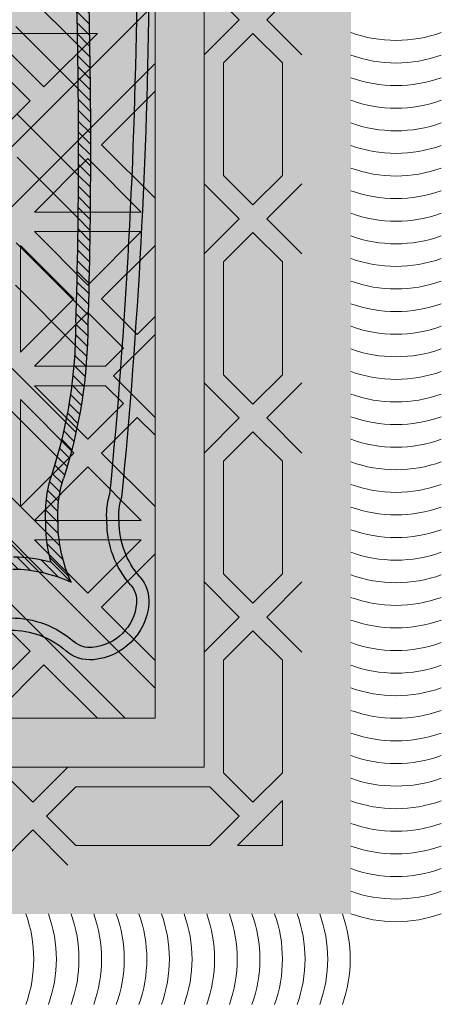
# Model space of a CAD drawing. Units: inches. Extents: x 844 to 2234, y 346 to 1084.
# Tile 29 of 93: x 1260.07 to 1265.57, y 682.93 to 695.76. Entities that reach past the tile are written whole.
import ezdxf

# ---------------------------------------------------------------- set-up
doc = ezdxf.new("R2010")
doc.units = ezdxf.units.IN
doc.header["$MEASUREMENT"] = 0
doc.layers.add('furniture', color=8, linetype='Continuous', lineweight=18)
doc.layers.add('RA-AP-01$0$INT', color=35, linetype='Continuous', lineweight=5)
doc.layers.add('RA-AP-01$0$FURN', color=3, linetype='Continuous')
doc.layers.add('RA-AP-01$0$WOOD', color=64, linetype='Continuous')

# ---------------------------------------------------------------- blocks, each defined once
blk = doc.blocks.new('A$C18D01794')
at = {"layer": 'RA-AP-01$0$INT'}
h = blk.add_hatch(color=256, dxfattribs=at)
h.paths.add_polyline_path([(4.3552, -6.1567), (4.3552, -8.0567), (5.4552, -8.0567), (5.4552, -6.1567)])
h.paths.add_polyline_path([(4.4052, -8.0067), (4.4052, -6.2067), (5.4052, -6.2067), (5.4052, -8.0067)], flags=16)
h = blk.add_hatch(color=256, dxfattribs=at)
h.paths.add_polyline_path([(4.4693, -7.0709), (4.5052, -7.035), (4.5052, -7.1067)])
h.paths.add_polyline_path([(4.4552, -7.085), (4.4769, -7.1067), (4.4335, -7.1067)])
h.paths.add_polyline_path([(4.4052, -7.035), (4.4411, -7.0709), (4.4052, -7.1067)])
h.paths.add_polyline_path([(4.4252, -6.9115), (4.4552, -6.8815), (4.4852, -6.9115), (4.4852, -7.0267), (4.4552, -7.0567), (4.4252, -7.0267)])
h.paths.add_polyline_path([(4.5052, -6.8315), (4.5052, -6.9032), (4.4693, -6.8673)])
h.paths.add_polyline_path([(4.4252, -6.7079), (4.4552, -6.6779), (4.4852, -6.7079), (4.4852, -6.8232), (4.4552, -6.8532), (4.4252, -6.8232)])
h.paths.add_polyline_path([(4.4252, -6.5044), (4.4552, -6.4744), (4.4852, -6.5044), (4.4852, -6.6196), (4.4552, -6.6496), (4.4252, -6.6196)])
h.paths.add_polyline_path([(4.4693, -6.6638), (4.5052, -6.6279), (4.5052, -6.6996)])
h.paths.add_polyline_path([(4.4052, -6.6279), (4.4411, -6.6638), (4.4052, -6.6996)])
h.paths.add_polyline_path([(4.4052, -6.4244), (4.4411, -6.4602), (4.4052, -6.4961)])
h.paths.add_polyline_path([(4.4693, -6.4602), (4.5052, -6.4244), (4.5052, -6.4961)])
h.paths.add_polyline_path([(4.4252, -6.3009), (4.4552, -6.2709), (4.4852, -6.3009), (4.4852, -6.4161), (4.4552, -6.4461), (4.4252, -6.4161)])
h.paths.add_polyline_path([(4.4252, -6.2267), (4.4711, -6.2267), (4.4252, -6.2726)])
h.paths.add_polyline_path([(4.4993, -6.2267), (4.6361, -6.2267), (4.6661, -6.2567), (4.6361, -6.2867), (4.4993, -6.2867), (4.4693, -6.2567)])
h.paths.add_polyline_path([(4.6802, -6.2709), (4.7161, -6.3067), (4.6443, -6.3067)])
h.paths.add_polyline_path([(4.6443, -6.2067), (4.7161, -6.2067), (4.6802, -6.2426)])
h.paths.add_polyline_path([(4.7243, -6.2267), (4.8611, -6.2267), (4.8911, -6.2567), (4.8611, -6.2867), (4.7243, -6.2867), (4.6943, -6.2567)])
h.paths.add_polyline_path([(4.9052, -6.2709), (4.9411, -6.3067), (4.8693, -6.3067)])
h.paths.add_polyline_path([(4.8693, -6.2067), (4.9411, -6.2067), (4.9052, -6.2426)])
h.paths.add_polyline_path([(4.9493, -6.2267), (5.0861, -6.2267), (5.1161, -6.2567), (5.0861, -6.2867), (4.9493, -6.2867), (4.9193, -6.2567)])
h.paths.add_polyline_path([(5.1302, -6.2709), (5.1661, -6.3067), (5.0943, -6.3067)])
h.paths.add_polyline_path([(5.0943, -6.2067), (5.1661, -6.2067), (5.1302, -6.2426)])
h.paths.add_polyline_path([(5.1743, -6.2267), (5.3111, -6.2267), (5.3411, -6.2567), (5.3111, -6.2867), (5.1743, -6.2867), (5.1443, -6.2567)])
h.paths.add_polyline_path([(5.3252, -6.3009), (5.3552, -6.2709), (5.3852, -6.3009), (5.3852, -6.4161), (5.3552, -6.4461), (5.3252, -6.4161)])
h.paths.add_polyline_path([(5.3393, -6.2267), (5.3852, -6.2267), (5.3852, -6.2726)])
h.paths.add_polyline_path([(5.3252, -6.5044), (5.3552, -6.4744), (5.3852, -6.5044), (5.3852, -6.6196), (5.3552, -6.6496), (5.3252, -6.6196)])
h.paths.add_polyline_path([(5.3052, -6.4244), (5.3411, -6.4602), (5.3052, -6.4961)])
h.paths.add_polyline_path([(5.3693, -6.4602), (5.4052, -6.4244), (5.4052, -6.4961)])
h.paths.add_polyline_path([(5.4052, -6.6279), (5.4052, -6.6996), (5.3693, -6.6638)])
h.paths.add_polyline_path([(5.3052, -6.6279), (5.3411, -6.6638), (5.3052, -6.6996)])
h.paths.add_polyline_path([(5.3252, -6.7079), (5.3552, -6.6779), (5.3852, -6.7079), (5.3852, -6.8232), (5.3552, -6.8532), (5.3252, -6.8232)])
h.paths.add_polyline_path([(5.3052, -6.8315), (5.3411, -6.8673), (5.3052, -6.9032)])
h.paths.add_polyline_path([(5.3252, -6.9115), (5.3552, -6.8815), (5.3852, -6.9115), (5.3852, -7.0267), (5.3552, -7.0567), (5.3252, -7.0267)])
h.paths.add_polyline_path([(5.4046, -6.8321, 0.001218), (5.4052, -6.8323), (5.4052, -6.9032), (5.3693, -6.8673)])
h.paths.add_polyline_path([(5.3693, -7.0709), (5.4052, -7.035), (5.4052, -7.1067)])
h.paths.add_polyline_path([(5.3552, -7.085), (5.3769, -7.1067), (5.3335, -7.1067)])
h.paths.add_polyline_path([(5.3052, -7.035), (5.3411, -7.0709), (5.3052, -7.1067)])
h = blk.add_hatch(color=256, dxfattribs=at)
h.paths.add_polyline_path([(4.5052, -6.6279), (4.4693, -6.6638), (4.5052, -6.6996), (4.5052, -6.8315), (4.4693, -6.8673), (4.5052, -6.9032), (4.5052, -7.035), (4.4693, -7.0709), (4.5052, -7.1067), (4.4769, -7.1067), (4.4552, -7.085), (4.4335, -7.1067), (4.4052, -7.1067), (4.4411, -7.0709), (4.4052, -7.035), (4.4052, -6.9032), (4.4411, -6.8673), (4.4052, -6.8315), (4.4052, -6.6996), (4.4411, -6.6638), (4.4052, -6.6279), (4.4052, -6.4961), (4.4411, -6.4602), (4.4052, -6.4244), (4.4052, -6.2067), (4.6443, -6.2067), (4.6802, -6.2426), (4.7161, -6.2067), (4.8693, -6.2067), (4.9052, -6.2426), (4.9411, -6.2067), (5.0943, -6.2067), (5.1302, -6.2426), (5.1661, -6.2067), (5.4052, -6.2067), (5.4052, -6.4244), (5.3693, -6.4602), (5.4052, -6.4961), (5.4052, -6.6279), (5.3693, -6.6638), (5.4052, -6.6996), (5.4052, -6.8315), (5.3693, -6.8673), (5.4052, -6.9032), (5.4052, -7.035), (5.3693, -7.0709), (5.4052, -7.1067), (5.3769, -7.1067), (5.3552, -7.085), (5.3335, -7.1067), (5.3052, -7.1067), (5.3411, -7.0709), (5.3052, -7.035), (5.3052, -6.9032), (5.3411, -6.8673), (5.3052, -6.8315), (5.3052, -6.6996), (5.3411, -6.6638), (5.3052, -6.6279), (5.3052, -6.4961), (5.3411, -6.4602), (5.3052, -6.4244), (5.3052, -6.3067), (5.1661, -6.3067), (5.1302, -6.2709), (5.0943, -6.3067), (4.9411, -6.3067), (4.9052, -6.2709), (4.8693, -6.3067), (4.7161, -6.3067), (4.6802, -6.2709), (4.6443, -6.3067), (4.5052, -6.3067), (4.5052, -6.4244), (4.4693, -6.4602), (4.5052, -6.4961)])
h.paths.add_polyline_path([(4.4852, -6.5044), (4.4552, -6.4744), (4.4252, -6.5044), (4.4252, -6.6196), (4.4552, -6.6496), (4.4852, -6.6196)], flags=16)
h.paths.add_polyline_path([(4.4552, -6.4461), (4.4852, -6.4161), (4.4852, -6.3009), (4.4552, -6.2709), (4.4252, -6.3009), (4.4252, -6.4161)], flags=16)
h.paths.add_polyline_path([(4.4552, -6.6779), (4.4252, -6.7079), (4.4252, -6.8232), (4.4552, -6.8532), (4.4852, -6.8232), (4.4852, -6.7079)], flags=16)
h.paths.add_polyline_path([(4.4993, -6.2867), (4.6361, -6.2867), (4.6661, -6.2567), (4.6361, -6.2267), (4.4993, -6.2267), (4.4693, -6.2567)], flags=16)
h.paths.add_polyline_path([(4.4252, -6.2726), (4.4711, -6.2267), (4.4252, -6.2267)], flags=16)
h.paths.add_polyline_path([(4.4552, -6.8815), (4.4252, -6.9115), (4.4252, -7.0267), (4.4552, -7.0567), (4.4852, -7.0267), (4.4852, -6.9115)], flags=16)
h.paths.add_polyline_path([(4.7243, -6.2867), (4.8611, -6.2867), (4.8911, -6.2567), (4.8611, -6.2267), (4.7243, -6.2267), (4.6943, -6.2567)], flags=16)
h.paths.add_polyline_path([(4.9193, -6.2567), (4.9493, -6.2867), (5.0861, -6.2867), (5.1161, -6.2567), (5.0861, -6.2267), (4.9493, -6.2267)], flags=16)
h.paths.add_polyline_path([(5.1443, -6.2567), (5.1743, -6.2867), (5.3111, -6.2867), (5.3411, -6.2567), (5.3111, -6.2267), (5.1743, -6.2267)], flags=16)
h.paths.add_polyline_path([(5.3252, -6.6196), (5.3552, -6.6496), (5.3852, -6.6196), (5.3852, -6.5044), (5.3552, -6.4744), (5.3252, -6.5044)], flags=16)
h.paths.add_polyline_path([(5.3252, -6.4161), (5.3552, -6.4461), (5.3852, -6.4161), (5.3852, -6.3009), (5.3552, -6.2709), (5.3252, -6.3009)], flags=16)
h.paths.add_polyline_path([(5.3252, -6.7079), (5.3252, -6.8232), (5.3552, -6.8532), (5.3852, -6.8232), (5.3852, -6.7079), (5.3552, -6.6779)], flags=16)
h.paths.add_polyline_path([(5.3252, -6.9115), (5.3252, -7.0267), (5.3552, -7.0567), (5.3852, -7.0267), (5.3852, -6.9115), (5.3552, -6.8815)], flags=16)
h.paths.add_polyline_path([(5.3393, -6.2267), (5.3852, -6.2726), (5.3852, -6.2267)], flags=16)
for points in [[(4.5052, -6.3067), (5.3052, -6.3067), (5.3052, -7.1067), (5.2552, -7.1067), (5.2552, -6.3567), (4.5552, -6.3567), (4.5552, -7.1067), (4.5052, -7.1067)], [(4.4052, -6.9032), (4.4411, -6.8673), (4.4052, -6.8315)]]:
    blk.add_hatch(color=256, dxfattribs=at).paths.add_polyline_path(points)
h = blk.add_hatch(color=256, dxfattribs=at)
h.paths.add_polyline_path([(4.5859, -6.3567), (4.5552, -6.3567), (4.5552, -6.3874), (4.8745, -6.7067), (4.9052, -6.676)])
h.paths.add_polyline_path([(5.2552, -6.3874), (5.2552, -6.3567), (5.2245, -6.3567), (4.9052, -6.676), (4.9359, -6.7067)])
h.paths.add_polyline_path([(4.9359, -6.7067), (4.9052, -6.7374), (5.2552, -7.0874), (5.2552, -7.026)])
h.paths.add_polyline_path([(4.5552, -7.026), (4.5552, -7.0874), (4.9052, -6.7374), (4.8745, -6.7067)])
h = blk.add_hatch(color=256, dxfattribs=at)
h.paths.add_polyline_path([(4.5859, -6.3567), (4.6142, -6.3567), (4.6688, -6.4114), (4.7235, -6.3567), (4.7718, -6.3567), (4.8264, -6.4114), (4.8628, -6.375), (4.8445, -6.3567), (4.8628, -6.3567), (4.9052, -6.3991), (4.9476, -6.3567), (4.9659, -6.3567), (4.9476, -6.375), (4.984, -6.4114), (5.0386, -6.3567), (5.0869, -6.3567), (5.1416, -6.4114), (5.1962, -6.3567), (5.2245, -6.3567), (4.9052, -6.676)])
h.paths.add_polyline_path([(4.8952, -6.6377), (4.8952, -6.5284), (4.8406, -6.5831)], flags=16)
h.paths.add_polyline_path([(4.9152, -6.6377), (4.9699, -6.5831), (4.9152, -6.5284)], flags=16)
h.paths.add_polyline_path([(4.8264, -6.5689), (4.8811, -6.5143), (4.7718, -6.5143)], flags=16)
h.paths.add_polyline_path([(4.984, -6.5689), (5.0386, -6.5143), (4.9293, -6.5143)], flags=16)
h.paths.add_polyline_path([(4.8811, -6.4943), (4.8264, -6.4396), (4.7718, -6.4943)], flags=16)
h.paths.add_polyline_path([(4.9293, -6.4943), (5.0386, -6.4943), (4.984, -6.4396)], flags=16)
h.paths.add_polyline_path([(4.8952, -6.4801), (4.8952, -6.4074), (4.8769, -6.3891), (4.8406, -6.4255)], flags=16)
h.paths.add_polyline_path([(4.9152, -6.4801), (4.9699, -6.4255), (4.9335, -6.3891), (4.9152, -6.4074)], flags=16)
h.paths.add_polyline_path([(4.7576, -6.4801), (4.8123, -6.4255), (4.7576, -6.3709)], flags=16)
h.paths.add_polyline_path([(4.7376, -6.4801), (4.7376, -6.3709), (4.683, -6.4255)], flags=16)
h.paths.add_polyline_path([(5.0528, -6.4801), (5.0528, -6.3709), (4.9981, -6.4255)], flags=16)
h.paths.add_polyline_path([(5.0728, -6.4801), (5.1274, -6.4255), (5.0728, -6.3709)], flags=16)
h.paths.add_polyline_path([(4.9359, -6.7067), (5.2552, -6.3874), (5.2552, -6.4157), (5.2006, -6.4704), (5.2552, -6.525), (5.2552, -6.5733), (5.2006, -6.6279), (5.2369, -6.6643), (5.2552, -6.646), (5.2552, -6.6643), (5.2128, -6.7067), (5.2552, -6.7491), (5.2552, -6.7674), (5.2369, -6.7491), (5.2006, -6.7855), (5.2552, -6.8401), (5.2552, -6.8884), (5.2006, -6.9431), (5.2552, -6.9977), (5.2552, -7.026)])
h.paths.add_polyline_path([(5.043, -6.7855), (5.0976, -6.8401), (5.0976, -6.7309)], flags=16)
h.paths.add_polyline_path([(5.0288, -6.7714), (5.0835, -6.7167), (4.9742, -6.7167)], flags=16)
h.paths.add_polyline_path([(5.1176, -6.8401), (5.1723, -6.7855), (5.1176, -6.7309)], flags=16)
h.paths.add_polyline_path([(5.0835, -6.6967), (5.0288, -6.6421), (4.9742, -6.6967)], flags=16)
h.paths.add_polyline_path([(5.1318, -6.8543), (5.1864, -6.7996), (5.2411, -6.8543)], flags=17)
h.paths.add_polyline_path([(5.1318, -6.7167), (5.1864, -6.7714), (5.2228, -6.735), (5.2045, -6.7167)], flags=16)
h.paths.add_polyline_path([(5.0976, -6.6826), (5.0976, -6.5733), (5.043, -6.6279)], flags=16)
h.paths.add_polyline_path([(5.1318, -6.8743), (5.2411, -6.8743), (5.1864, -6.9289)], flags=17)
h.paths.add_polyline_path([(5.1318, -6.6967), (5.2045, -6.6967), (5.2228, -6.6784), (5.1864, -6.6421)], flags=16)
h.paths.add_polyline_path([(5.1176, -6.6826), (5.1723, -6.6279), (5.1176, -6.5733)], flags=16)
h.paths.add_polyline_path([(5.1864, -6.6138), (5.2411, -6.5591), (5.1318, -6.5591)], flags=16)
h.paths.add_polyline_path([(5.1318, -6.5391), (5.2411, -6.5391), (5.1864, -6.4845)], flags=16)
h.paths.add_polyline_path([(5.2552, -7.0874), (5.2552, -7.1067), (4.5552, -7.1067), (4.5552, -7.0874), (4.9052, -6.7374)])
h.paths.add_polyline_path([(4.984, -6.8445), (4.9293, -6.8991), (5.0386, -6.8991)], flags=16)
h.paths.add_polyline_path([(4.9699, -6.8304), (4.9152, -6.7757), (4.9152, -6.885)], flags=16)
h.paths.add_polyline_path([(4.9293, -6.9191), (4.984, -6.9738), (5.0386, -6.9191)], flags=16)
h.paths.add_polyline_path([(5.0528, -6.9333), (4.9981, -6.9879), (5.0528, -7.0426)], flags=16)
h.paths.add_polyline_path([(5.0728, -6.9333), (5.0728, -7.0426), (5.1274, -6.9879)], flags=16)
h.paths.add_polyline_path([(4.8952, -6.7757), (4.8406, -6.8304), (4.8952, -6.885)], flags=16)
h.paths.add_polyline_path([(4.9152, -6.9333), (4.9152, -7.006), (4.9335, -7.0243), (4.9699, -6.9879)], flags=16)
h.paths.add_polyline_path([(4.8811, -6.8991), (4.8264, -6.8445), (4.7718, -6.8991)], flags=16)
h.paths.add_polyline_path([(4.8952, -6.9333), (4.8406, -6.9879), (4.8769, -7.0243), (4.8952, -7.006)], flags=16)
h.paths.add_polyline_path([(4.984, -7.0021), (4.9476, -7.0384), (4.9659, -7.0567), (5.0386, -7.0567)], flags=16)
h.paths.add_polyline_path([(4.8811, -6.9191), (4.7718, -6.9191), (4.8264, -6.9738)], flags=16)
h.paths.add_polyline_path([(4.9052, -7.0143), (4.8628, -7.0567), (4.9476, -7.0567)], flags=16)
h.paths.add_polyline_path([(5.1416, -7.0021), (5.0869, -7.0567), (5.1962, -7.0567)], flags=16)
h.paths.add_polyline_path([(4.8264, -7.0021), (4.7718, -7.0567), (4.8445, -7.0567), (4.8628, -7.0384)], flags=16)
h.paths.add_polyline_path([(4.8123, -6.9879), (4.7576, -6.9333), (4.7576, -7.0426)], flags=16)
h.paths.add_polyline_path([(4.7376, -6.9333), (4.683, -6.9879), (4.7376, -7.0426)], flags=16)
h.paths.add_polyline_path([(4.7235, -7.0567), (4.6688, -7.0021), (4.6142, -7.0567)], flags=16)
h.paths.add_polyline_path([(4.5976, -6.7067), (4.5552, -6.6643), (4.5552, -6.646), (4.5735, -6.6643), (4.6099, -6.6279), (4.5552, -6.5733), (4.5552, -6.525), (4.6099, -6.4704), (4.5552, -6.4157), (4.5552, -6.3874), (4.8745, -6.7067), (4.5552, -7.026), (4.5552, -6.9977), (4.6099, -6.9431), (4.5552, -6.8884), (4.5552, -6.8401), (4.6099, -6.7855), (4.5735, -6.7491), (4.5552, -6.7674), (4.5552, -6.7491)])
h.paths.add_polyline_path([(4.7128, -6.7309), (4.7128, -6.8401), (4.7674, -6.7855)], flags=16)
h.paths.add_polyline_path([(4.7269, -6.7167), (4.7816, -6.7714), (4.8362, -6.7167)], flags=16)
h.paths.add_polyline_path([(4.6928, -6.7309), (4.6381, -6.7855), (4.6928, -6.8401)], flags=16)
h.paths.add_polyline_path([(4.7269, -6.6967), (4.8362, -6.6967), (4.7816, -6.6421)], flags=16)
h.paths.add_polyline_path([(4.6786, -6.7167), (4.6059, -6.7167), (4.5876, -6.735), (4.624, -6.7714)], flags=16)
h.paths.add_polyline_path([(4.7128, -6.6826), (4.7674, -6.6279), (4.7128, -6.5733)], flags=16)
h.paths.add_polyline_path([(4.6786, -6.6967), (4.624, -6.6421), (4.5876, -6.6784), (4.6059, -6.6967)], flags=16)
h.paths.add_polyline_path([(4.6928, -6.6826), (4.6928, -6.5733), (4.6381, -6.6279)], flags=16)
h.paths.add_polyline_path([(4.624, -6.7996), (4.6786, -6.8543), (4.5693, -6.8543)], flags=17)
h.paths.add_polyline_path([(4.624, -6.6138), (4.6786, -6.5591), (4.5693, -6.5591)], flags=16)
h.paths.add_polyline_path([(4.6786, -6.8743), (4.624, -6.9289), (4.5693, -6.8743)], flags=17)
h.paths.add_polyline_path([(4.6786, -6.5391), (4.624, -6.4845), (4.5693, -6.5391)], flags=16)
h = blk.add_hatch(color=256, dxfattribs=at)
h.paths.add_polyline_path([(4.9699, -6.5831), (4.9152, -6.6377), (4.9152, -6.5284)])
h.paths.add_polyline_path([(4.8952, -6.6377), (4.8406, -6.5831), (4.8952, -6.5284)])
h.paths.add_polyline_path([(4.8264, -6.5689), (4.7718, -6.5143), (4.8811, -6.5143)])
h.paths.add_polyline_path([(4.8811, -6.4943), (4.7718, -6.4943), (4.8264, -6.4396)])
h.paths.add_polyline_path([(4.8952, -6.4801), (4.8406, -6.4255), (4.8769, -6.3891), (4.8952, -6.4074)])
h.paths.add_polyline_path([(4.8628, -6.375), (4.8264, -6.4114), (4.7718, -6.3567), (4.8445, -6.3567)])
h.paths.add_polyline_path([(4.8123, -6.4255), (4.7576, -6.4801), (4.7576, -6.3709)])
h.paths.add_polyline_path([(4.7376, -6.4801), (4.683, -6.4255), (4.7376, -6.3709)])
h.paths.add_polyline_path([(4.6688, -6.4114), (4.6142, -6.3567), (4.7235, -6.3567)])
h.paths.add_polyline_path([(4.9052, -6.3991), (4.8628, -6.3567), (4.9476, -6.3567)])
h.paths.add_polyline_path([(4.9152, -6.4801), (4.9152, -6.4074), (4.9335, -6.3891), (4.9699, -6.4255)])
h.paths.add_polyline_path([(5.0386, -6.4943), (4.9293, -6.4943), (4.984, -6.4396)])
h.paths.add_polyline_path([(4.984, -6.5689), (4.9293, -6.5143), (5.0386, -6.5143)])
h.paths.add_polyline_path([(5.0528, -6.4801), (4.9981, -6.4255), (5.0528, -6.3709)])
h.paths.add_polyline_path([(4.984, -6.4114), (4.9476, -6.375), (4.9659, -6.3567), (5.0386, -6.3567)])
h.paths.add_polyline_path([(5.1274, -6.4255), (5.0728, -6.4801), (5.0728, -6.3709)])
h.paths.add_polyline_path([(5.1416, -6.4114), (5.0869, -6.3567), (5.1962, -6.3567)])
h = blk.add_hatch(color=256, dxfattribs=at)
h.paths.add_polyline_path([(4.7816, -6.7714), (4.8362, -6.7167), (4.7269, -6.7167)])
h.paths.add_polyline_path([(4.8362, -6.6967), (4.7816, -6.6421), (4.7269, -6.6967)])
h.paths.add_polyline_path([(4.7674, -6.6279), (4.7128, -6.5733), (4.7128, -6.6826)])
h.paths.add_polyline_path([(4.6928, -6.6826), (4.6928, -6.5733), (4.6381, -6.6279)])
h.paths.add_polyline_path([(4.6786, -6.6967), (4.624, -6.6421), (4.5876, -6.6784), (4.6059, -6.6967)])
h.paths.add_polyline_path([(4.5735, -6.6643), (4.6099, -6.6279), (4.5552, -6.5733), (4.5552, -6.646)])
h.paths.add_polyline_path([(4.624, -6.6138), (4.6786, -6.5591), (4.5693, -6.5591)])
h.paths.add_polyline_path([(4.6786, -6.5391), (4.624, -6.4845), (4.5693, -6.5391)])
h.paths.add_polyline_path([(4.6099, -6.4704), (4.5552, -6.4157), (4.5552, -6.525)])
h.paths.add_polyline_path([(4.5976, -6.7067), (4.5552, -6.6643), (4.5552, -6.7491)])
h.paths.add_polyline_path([(4.6786, -6.7167), (4.6059, -6.7167), (4.5876, -6.735), (4.624, -6.7714)])
h.paths.add_polyline_path([(4.6928, -6.8401), (4.6928, -6.7309), (4.6381, -6.7855)])
h.paths.add_polyline_path([(4.7674, -6.7855), (4.7128, -6.7309), (4.7128, -6.8401)])
h.paths.add_polyline_path([(4.6786, -6.8543), (4.624, -6.7996), (4.5693, -6.8543)])
h.paths.add_polyline_path([(4.6099, -6.7855), (4.5735, -6.7491), (4.5552, -6.7674), (4.5552, -6.8401)])
h.paths.add_polyline_path([(4.624, -6.9289), (4.6786, -6.8743), (4.5693, -6.8743)])
h.paths.add_polyline_path([(4.6099, -6.9431), (4.5552, -6.8884), (4.5552, -6.9977)])
h = blk.add_hatch(color=256, dxfattribs=at)
h.paths.add_polyline_path([(4.8952, -6.7757), (4.8406, -6.8304), (4.8952, -6.885)])
h.paths.add_polyline_path([(4.9152, -6.885), (4.9699, -6.8304), (4.9152, -6.7757)])
h.paths.add_polyline_path([(5.0386, -6.8991), (4.984, -6.8445), (4.9293, -6.8991)])
h.paths.add_polyline_path([(4.9293, -6.9191), (4.984, -6.9738), (5.0386, -6.9191)])
h.paths.add_polyline_path([(4.9152, -6.9333), (4.9152, -7.006), (4.9335, -7.0243), (4.9699, -6.9879)])
h.paths.add_polyline_path([(5.0386, -7.0567), (4.984, -7.0021), (4.9476, -7.0384), (4.9659, -7.0567)])
h.paths.add_polyline_path([(5.0528, -7.0426), (5.0528, -6.9333), (4.9981, -6.9879)])
h.paths.add_polyline_path([(5.0728, -7.0426), (5.1274, -6.9879), (5.0728, -6.9333)])
h.paths.add_polyline_path([(5.1416, -7.0021), (5.0869, -7.0567), (5.1962, -7.0567)])
h.paths.add_polyline_path([(4.9476, -7.0567), (4.9052, -7.0143), (4.8628, -7.0567)])
h.paths.add_polyline_path([(4.8406, -6.9879), (4.8769, -7.0243), (4.8952, -7.006), (4.8952, -6.9333)])
h.paths.add_polyline_path([(4.8811, -6.9191), (4.7718, -6.9191), (4.8264, -6.9738)])
h.paths.add_polyline_path([(4.8811, -6.8991), (4.8264, -6.8445), (4.7718, -6.8991)])
h.paths.add_polyline_path([(4.7576, -7.0426), (4.8123, -6.9879), (4.7576, -6.9333)])
h.paths.add_polyline_path([(4.8264, -7.0021), (4.7718, -7.0567), (4.8445, -7.0567), (4.8628, -7.0384)])
h.paths.add_polyline_path([(4.7376, -7.0426), (4.7376, -6.9333), (4.683, -6.9879)])
h.paths.add_polyline_path([(4.6688, -7.0021), (4.6142, -7.0567), (4.7235, -7.0567)])
for p, q in [((4.6443, -6.2067), (4.6802, -6.2426)), ((4.7161, -6.2067), (4.6802, -6.2426)), ((4.4711, -6.2267), (4.4252, -6.2726)), ((4.4252, -6.2726), (4.4252, -6.2267)), ((4.4711, -6.2267), (4.4252, -6.2267)), ((4.4993, -6.2267), (4.4693, -6.2567)), ((4.6361, -6.2267), (4.4993, -6.2267)), ((4.6361, -6.2267), (4.6661, -6.2567)), ((4.4993, -6.2867), (4.4693, -6.2567)), ((4.6361, -6.2867), (4.6661, -6.2567)), ((4.4252, -6.3009), (4.4552, -6.2709)), ((4.4852, -6.3009), (4.4552, -6.2709)), ((4.6443, -6.3067), (4.6802, -6.2709)), ((4.7161, -6.3067), (4.6802, -6.2709)), ((4.6361, -6.2867), (4.4993, -6.2867)), ((4.4252, -6.4161), (4.4252, -6.3009)), ((4.4852, -6.3009), (4.4852, -6.4161)), ((5.2672, -6.3067), (4.5432, -6.3067)), ((5.2672, -6.3067), (4.5432, -6.3067)), ((4.5552, -6.3567), (5.2552, -6.3567)), ((4.5552, -7.1067), (4.5552, -6.3567)), ((4.9052, -6.676), (4.5859, -6.3567)), ((4.6142, -6.3567), (4.6688, -6.4114)), ((4.7235, -6.3567), (4.6688, -6.4114)), ((4.7376, -6.3709), (4.683, -6.4255)), ((4.8745, -6.7067), (4.5552, -6.3874)), ((4.4552, -6.4461), (4.4252, -6.4161)), ((4.4552, -6.4461), (4.4852, -6.4161)), ((4.5552, -6.4157), (4.6099, -6.4704)), ((4.4411, -6.4602), (4.4052, -6.4244)), ((4.4693, -6.4602), (4.5052, -6.4244)), ((4.683, -6.4255), (4.7376, -6.4801)), ((4.4052, -6.4961), (4.4411, -6.4602)), ((4.5052, -6.4961), (4.4693, -6.4602)), ((4.5552, -6.525), (4.6099, -6.4704)), ((4.4252, -6.5044), (4.4552, -6.4744)), ((4.4852, -6.5044), (4.4552, -6.4744)), ((4.5693, -6.5391), (4.624, -6.4845)), ((4.624, -6.4845), (4.6786, -6.5391)), ((4.4252, -6.6196), (4.4252, -6.5044)), ((4.4852, -6.6196), (4.4852, -6.5044)), ((4.6786, -6.5391), (4.5693, -6.5391)), ((4.5693, -6.5591), (4.624, -6.6138)), ((4.6786, -6.5591), (4.5693, -6.5591)), ((4.6786, -6.5591), (4.624, -6.6138)), ((4.5552, -6.646), (4.5552, -6.5733)), ((4.5552, -6.5733), (4.6099, -6.6279)), ((4.6928, -6.5733), (4.6381, -6.6279)), ((4.6928, -6.5733), (4.6928, -6.6826)), ((4.4252, -6.6196), (4.4552, -6.6496)), ((4.4852, -6.6196), (4.4552, -6.6496)), ((4.4052, -6.6279), (4.4411, -6.6638)), ((4.5052, -6.6279), (4.4693, -6.6638)), ((4.6099, -6.6279), (4.5735, -6.6643)), ((4.6928, -6.6826), (4.6381, -6.6279)), ((4.624, -6.6421), (4.5876, -6.6784)), ((4.6786, -6.6967), (4.624, -6.6421)), ((4.5552, -6.646), (4.5735, -6.6643)), ((4.4052, -6.6996), (4.4411, -6.6638)), ((4.5052, -6.6996), (4.4693, -6.6638)), ((4.5552, -6.7491), (4.5552, -6.6643)), ((4.5976, -6.7067), (4.5552, -6.6643)), ((4.4252, -6.7079), (4.4552, -6.6779)), ((4.4852, -6.7079), (4.4552, -6.6779)), ((4.6059, -6.6967), (4.5876, -6.6784)), ((4.6059, -6.6967), (4.6786, -6.6967)), ((4.4252, -6.8232), (4.4252, -6.7079)), ((4.4852, -6.8232), (4.4852, -6.7079)), ((4.8745, -6.7067), (4.5552, -7.026)), ((4.5976, -6.7067), (4.5552, -6.7491)), ((4.6059, -6.7167), (4.5876, -6.735)), ((4.6059, -6.7167), (4.6786, -6.7167)), ((4.6786, -6.7167), (4.624, -6.7714)), ((4.6928, -6.7309), (4.6381, -6.7855)), ((4.6928, -6.8401), (4.6928, -6.7309)), ((4.9052, -6.7374), (4.5552, -7.0874)), ((4.624, -6.7714), (4.5876, -6.735)), ((4.5735, -6.7491), (4.5552, -6.7674)), ((4.5552, -6.7674), (4.5735, -6.7491)), ((4.6099, -6.7855), (4.5735, -6.7491)), ((4.5552, -6.7674), (4.5552, -6.8401)), ((4.5552, -6.8401), (4.6099, -6.7855)), ((4.6928, -6.8401), (4.6381, -6.7855)), ((4.5693, -6.8543), (4.624, -6.7996)), ((4.6786, -6.8543), (4.624, -6.7996)), ((4.4252, -6.8232), (4.4552, -6.8532)), ((4.4852, -6.8232), (4.4552, -6.8532)), ((4.4052, -6.8315), (4.4411, -6.8673)), ((4.5052, -6.8315), (4.4693, -6.8673)), ((4.6786, -6.8543), (4.5693, -6.8543)), ((4.4052, -6.9032), (4.4411, -6.8673)), ((4.5052, -6.9032), (4.4693, -6.8673)), ((4.5693, -6.8743), (4.624, -6.9289)), ((4.6786, -6.8743), (4.5693, -6.8743)), ((4.624, -6.9289), (4.6786, -6.8743)), ((4.4252, -6.9115), (4.4552, -6.8815)), ((4.4852, -6.9115), (4.4552, -6.8815)), ((4.5552, -6.8884), (4.6099, -6.9431)), ((4.5552, -6.8884), (4.5552, -6.9977)), ((4.4252, -6.9115), (4.4252, -7.0267)), ((4.4852, -6.9115), (4.4852, -7.0267)), ((4.683, -6.9879), (4.7376, -6.9333)), ((4.5552, -6.9977), (4.6099, -6.9431)), ((4.7376, -7.0426), (4.683, -6.9879)), ((4.6142, -7.0567), (4.6688, -7.0021)), ((4.7235, -7.0567), (4.6688, -7.0021)), ((4.4052, -7.035), (4.4411, -7.0709)), ((4.4252, -7.0267), (4.4552, -7.0567)), ((4.4852, -7.0267), (4.4552, -7.0567)), ((4.5052, -7.035), (4.4693, -7.0709)), ((4.7235, -7.0567), (4.6142, -7.0567)), ((4.4411, -7.0709), (4.4052, -7.1067)), ((4.4693, -7.0709), (4.5052, -7.1067))]:
    blk.add_line(p, q, dxfattribs=at)
blk.add_lwpolyline([(5.3052, -7.1067), (5.3052, -6.3067), (4.5052, -6.3067), (4.5052, -7.1067)], dxfattribs=at)
for centre, start, end in [((4.4922, -6.1105), 160.2038, 199.7962), ((4.5153, -6.1105), 160.2038, 199.7962), ((4.5384, -6.1105), 160.2038, 199.7962), ((4.5615, -6.1105), 160.2038, 199.7962), ((4.5846, -6.1105), 160.2038, 199.7962), ((4.6077, -6.1105), 160.2038, 199.7962), ((4.6308, -6.1105), 160.2038, 199.7962), ((4.6539, -6.1105), 160.2038, 199.7962), ((4.677, -6.1105), 160.2038, 199.7962), ((4.7001, -6.1105), 160.2038, 199.7962), ((4.7232, -6.1105), 160.2038, 199.7962), ((4.7463, -6.1105), 160.2038, 199.7962), ((4.7694, -6.1105), 160.2038, 199.7962), ((4.7925, -6.1105), 160.2038, 199.7962), ((4.8156, -6.1105), 160.2038, 199.7962), ((4.309, -6.2852), 70.2038, 109.7962), ((4.309, -6.3083), 70.2038, 109.7962), ((4.309, -6.3314), 70.2038, 109.7962), ((4.309, -6.3545), 70.2038, 109.7962), ((4.309, -6.3776), 70.2038, 109.7962), ((4.309, -6.4007), 70.2038, 109.7962), ((4.309, -6.4238), 70.2038, 109.7962), ((4.309, -6.4469), 70.2038, 109.7962), ((4.309, -6.47), 70.2038, 109.7962), ((4.309, -6.4931), 70.2038, 109.7962), ((4.309, -6.5162), 70.2038, 109.7962), ((4.309, -6.5393), 70.2038, 109.7962), ((4.309, -6.5624), 70.2038, 109.7962), ((4.309, -6.5855), 70.2038, 109.7962), ((4.309, -6.6086), 70.2038, 109.7962), ((4.309, -6.6317), 70.2038, 109.7962), ((4.309, -6.6548), 70.2038, 109.7962), ((4.309, -6.6779), 70.2038, 109.7962), ((4.309, -6.701), 70.2038, 109.7962), ((4.309, -6.7241), 70.2038, 109.7962), ((4.309, -6.7472), 70.2038, 109.7962), ((4.309, -6.7703), 70.2038, 109.7962), ((4.309, -6.7934), 70.2038, 109.7962), ((4.309, -6.7934), 70.2038, 109.7962), ((4.309, -6.8165), 70.2038, 109.7962), ((4.309, -6.8396), 70.2038, 109.7962), ((4.309, -6.8627), 70.2038, 109.7962), ((4.309, -6.8858), 70.2038, 109.7962), ((4.309, -6.9089), 70.2038, 109.7962), ((4.309, -6.932), 70.2038, 109.7962), ((4.309, -6.9551), 70.2038, 109.7962), ((4.309, -6.9782), 70.2038, 109.7962), ((4.309, -7.0013), 70.2038, 109.7962), ((4.309, -7.0244), 70.2038, 109.7962), ((4.309, -7.0475), 70.2038, 109.7962), ((4.309, -7.0706), 70.2038, 109.7962), ((4.309, -7.0937), 70.2038, 109.7962), ((4.309, -7.1168), 70.2038, 109.7962), ((4.309, -7.1399), 70.2038, 109.7962), ((4.309, -7.163), 70.2038, 109.7962), ((4.309, -7.1861), 70.2038, 109.7962)]:
    blk.add_arc(centre, 0.1364, start, end, dxfattribs=at)
blk = doc.blocks.new('A$C32926AE1')
at = {"layer": 'RA-AP-01$0$WOOD'}
h = blk.add_hatch(color=256, dxfattribs=at)
h.dxf.hatch_style = 1
h.paths.add_polyline_path([(5.15743, 4.57348, -0.100949), (5.1554, 4.59337, -0.184266), (5.17225, 4.6388, 0.205661), (5.17956, 4.66132, 0.361434), (5.13435, 4.70652, 0.205661), (5.11183, 4.69921, -0.184266), (5.0664, 4.68237, -0.105531), (5.04566, 4.68467, 0.156764), (4.76389, 4.68467, -0.105531), (4.74314, 4.68237, -0.184266), (4.69771, 4.69921, 0.205661), (4.67519, 4.70652, 0.361434), (4.62998, 4.66132, 0.205661), (4.63729, 4.6388, -0.184266), (4.65414, 4.59337, -0.100949), (4.65211, 4.57348, 0.02141), (4.62975, 4.15671, 0.02141), (4.65211, 3.73994, -0.100949), (4.65414, 3.72006, -0.184266), (4.63729, 3.67463, 0.205661), (4.62998, 3.65211, 0.361434), (4.67519, 3.6069, 0.205661), (4.69771, 3.61421, -0.184266), (4.74314, 3.63106, -0.105531), (4.76389, 3.62875, 0.156764), (5.04566, 3.62875, -0.105531), (5.0664, 3.63106, -0.184266), (5.11183, 3.61421, 0.205661), (5.13435, 3.6069, 0.361434), (5.17956, 3.65211, 0.205661), (5.17225, 3.67463, -0.184266), (5.1554, 3.72006, -0.100949), (5.15743, 3.73994, 0.02141), (5.17979, 4.15671, 0.02141)])
h.paths.add_polyline_path([(4.63975, 4.15671, 0.021354), (4.66197, 3.74189, -0.094076), (4.66414, 3.71961, -0.182482), (4.64481, 3.66804, 0.205661), (4.63994, 3.65302, 0.361434), (4.67611, 3.61686, 0.205661), (4.69112, 3.62173, -0.182482), (4.7427, 3.64106, -0.102989), (4.76699, 3.63826, 0.156709), (5.04255, 3.63826, -0.102989), (5.06685, 3.64106, -0.182482), (5.11842, 3.62173, 0.205661), (5.13344, 3.61686, 0.361434), (5.1696, 3.65302, 0.205661), (5.16473, 3.66804, -0.182482), (5.1454, 3.71961, -0.094076), (5.14757, 3.74189, 0.021354), (5.16979, 4.15671, 0.021354), (5.14757, 4.57154, -0.094076), (5.1454, 4.59381, -0.182482), (5.16473, 4.64539, 0.205661), (5.1696, 4.6604, 0.361434), (5.13344, 4.69657, 0.205661), (5.11842, 4.69169, -0.182482), (5.06685, 4.67236, -0.102989), (5.04255, 4.67517, 0.156709), (4.76699, 4.67517, -0.102989), (4.7427, 4.67236, -0.182482), (4.69112, 4.69169, 0.205661), (4.67611, 4.69657, 0.361434), (4.63994, 4.6604, 0.205661), (4.64481, 4.64539, -0.182482), (4.66414, 4.59381, -0.094076), (4.66197, 4.57154, 0.021354)], flags=16)
h.paths.add_polyline_path([(5.12979, 4.43217, -0.014166), (5.13015, 4.15693, -0.014166), (5.12979, 3.88169, -0.078525), (5.1098, 3.75514, 0.094597), (5.10541, 3.7179, 0.104317), (5.11607, 3.67039, 0.104317), (5.06856, 3.68105, 0.094597), (5.03132, 3.67666, -0.158024), (4.77823, 3.67666, 0.094597), (4.74098, 3.68105, 0.104317), (4.69347, 3.67039, 0.104317), (4.70413, 3.7179, 0.094597), (4.69975, 3.75514, -0.078525), (4.67975, 3.88169, -0.014166), (4.67939, 4.15693, -0.014166), (4.67975, 4.43217, -0.078525), (4.69975, 4.55871, 0.094597), (4.70413, 4.59596, 0.104317), (4.69347, 4.64347, 0.104317), (4.74098, 4.6328, 0.094597), (4.77823, 4.63719, -0.158024), (5.03132, 4.63719, 0.094597), (5.06856, 4.6328, 0.104317), (5.11607, 4.64347, 0.104317), (5.10541, 4.59596, 0.094597), (5.1098, 4.55871, -0.078525)], flags=0)
h.paths.add_polyline_path([(5.11979, 4.43226, -0.0142), (5.12016, 4.15693, -0.0142), (5.11979, 3.8816, -0.078489), (5.10027, 3.75819, 0.094014), (5.09541, 3.71748, 0.060627), (5.09962, 3.68684, 0.060627), (5.06898, 3.69105, 0.094014), (5.02827, 3.68619, -0.158071), (4.78127, 3.68619, 0.094014), (4.74056, 3.69105, 0.060627), (4.70993, 3.68684, 0.060627), (4.71413, 3.71748, 0.094014), (4.70927, 3.75819, -0.078489), (4.68975, 3.8816, -0.0142), (4.68939, 4.15693, -0.0142), (4.68975, 4.43226, -0.078489), (4.70927, 4.55566, 0.094014), (4.71413, 4.59638, 0.060627), (4.70993, 4.62701, 0.060627), (4.74056, 4.62281, 0.094014), (4.78127, 4.62767, -0.158071), (5.02827, 4.62767, 0.094014), (5.06898, 4.62281, 0.060627), (5.09962, 4.62701, 0.060627), (5.09541, 4.59638, 0.094014), (5.10027, 4.55566, -0.078489)], flags=0)
h.paths.add_polyline_path([(5.06979, 4.43022, -0.014242), (5.07017, 4.15693, -0.014242), (5.06979, 3.88364, -0.080061), (5.05266, 3.77346, 0.052642), (5.04591, 3.74055, 0.052642), (5.013, 3.7338, -0.158303), (4.79655, 3.7338, 0.052642), (4.76363, 3.74055, 0.052642), (4.75688, 3.77346, -0.080061), (4.73975, 3.88364, -0.014242), (4.73937, 4.15693, -0.014242), (4.73975, 4.43022, -0.080061), (4.75688, 4.54039, 0.052642), (4.76363, 4.5733, 0.052642), (4.79655, 4.58006, -0.158303), (5.013, 4.58006, 0.052642), (5.04591, 4.5733, 0.052642), (5.05266, 4.54039, -0.080061)], flags=0)
h.paths.add_polyline_path([(5.04979, 4.43038, -0.01431), (5.05018, 4.15693, -0.01431), (5.04979, 3.88347, -0.080069), (5.03362, 3.77958, 0.030626), (5.02824, 3.75822, 0.030626), (5.00688, 3.75284, -0.158398), (4.80266, 3.75284, 0.030626), (4.7813, 3.75822, 0.030626), (4.77592, 3.77958, -0.080069), (4.75975, 3.88347, -0.01431), (4.75936, 4.15693, -0.01431), (4.75975, 4.43038, -0.080069), (4.77592, 4.53427, 0.030626), (4.7813, 4.55564, 0.030626), (4.80266, 4.56102, -0.158398), (5.00688, 4.56102, 0.030626), (5.02824, 4.55564, 0.030626), (5.03362, 4.53427, -0.080069)], flags=0)
h.paths.add_polyline_path([(4.99977, 4.42817, -0.014344), (5.0002, 4.15693, -0.014344), (4.99977, 3.88568, -0.078464), (4.98736, 3.7991, -0.150605), (4.82219, 3.7991, -0.078464), (4.80978, 3.88568, -0.014344), (4.80934, 4.15693, -0.014344), (4.80978, 4.42817, -0.078464), (4.82219, 4.51475, -0.150605), (4.98736, 4.51475, -0.078464)], flags=0)
h.paths.add_polyline_path([(4.97976, 4.42764, -0.014377), (4.98021, 4.15693, -0.014377), (4.97976, 3.88621, -0.068924), (4.97118, 3.81528, -0.129665), (4.83836, 3.81528, -0.068924), (4.82979, 3.88621, -0.014377), (4.82934, 4.15693, -0.014377), (4.82979, 4.42764, -0.068924), (4.83836, 4.49858, -0.129665), (4.97118, 4.49858, -0.068924)], flags=0)
h = blk.add_hatch(color=256, dxfattribs=at)
h.dxf.hatch_style = 1
h.paths.add_polyline_path([(5.1454, 4.59381, -0.182482), (5.16473, 4.64539, 0.205661), (5.1696, 4.6604, 0.361434), (5.13344, 4.69657, 0.205661), (5.11842, 4.69169, -0.182482), (5.06685, 4.67236, -0.102989), (5.04255, 4.67517, 0.156709), (4.76699, 4.67517, -0.102989), (4.7427, 4.67236, -0.182482), (4.69112, 4.69169, 0.205661), (4.67611, 4.69657, 0.361434), (4.63994, 4.6604, 0.205661), (4.64481, 4.64539, -0.182482), (4.66414, 4.59381, -0.094076), (4.66197, 4.57154, 0.021354), (4.63975, 4.15671, 0.021354), (4.66197, 3.74189, -0.094076), (4.66414, 3.71961, -0.182482), (4.64481, 3.66804, 0.205661), (4.63994, 3.65302, 0.361434), (4.67611, 3.61686, 0.205661), (4.69112, 3.62173, -0.182482), (4.7427, 3.64106, -0.102989), (4.76699, 3.63826, 0.156709), (5.04255, 3.63826, -0.102989), (5.06685, 3.64106, -0.182482), (5.11842, 3.62173, 0.205661), (5.13344, 3.61686, 0.361434), (5.1696, 3.65302, 0.205661), (5.16473, 3.66804, -0.182482), (5.1454, 3.71961, -0.094076), (5.14757, 3.74189, 0.021354), (5.16979, 4.15671, 0.021354), (5.14757, 4.57154, -0.094076)])
h.paths.add_polyline_path([(5.1098, 4.55871, -0.078525), (5.12979, 4.43217, -0.014166), (5.13015, 4.15693, -0.014166), (5.12979, 3.88169, -0.078525), (5.1098, 3.75514, 0.094597), (5.10541, 3.7179, 0.104317), (5.11607, 3.67039, 0.104317), (5.06856, 3.68105, 0.094597), (5.03132, 3.67666, -0.158024), (4.77823, 3.67666, 0.094597), (4.74098, 3.68105, 0.104317), (4.69347, 3.67039, 0.104317), (4.70413, 3.7179, 0.094597), (4.69975, 3.75514, -0.078525), (4.67975, 3.88169, -0.014166), (4.67939, 4.15693, -0.014166), (4.67975, 4.43217, -0.078525), (4.69975, 4.55871, 0.094597), (4.70413, 4.59596, 0.104317), (4.69347, 4.64347, 0.104317), (4.74098, 4.6328, 0.094597), (4.77823, 4.63719, -0.158024), (5.03132, 4.63719, 0.094597), (5.06856, 4.6328, 0.104317), (5.11607, 4.64347, 0.104317), (5.10541, 4.59596, 0.094597)], flags=16)
h.paths.add_polyline_path([(5.10027, 4.55566, -0.078489), (5.11979, 4.43226, -0.0142), (5.12016, 4.15693, -0.0142), (5.11979, 3.8816, -0.078489), (5.10027, 3.75819, 0.094014), (5.09541, 3.71748, 0.060627), (5.09962, 3.68684, 0.060627), (5.06898, 3.69105, 0.094014), (5.02827, 3.68619, -0.158071), (4.78127, 3.68619, 0.094014), (4.74056, 3.69105, 0.060627), (4.70993, 3.68684, 0.060627), (4.71413, 3.71748, 0.094014), (4.70927, 3.75819, -0.078489), (4.68975, 3.8816, -0.0142), (4.68939, 4.15693, -0.0142), (4.68975, 4.43226, -0.078489), (4.70927, 4.55566, 0.094014), (4.71413, 4.59638, 0.060627), (4.70993, 4.62701, 0.060627), (4.74056, 4.62281, 0.094014), (4.78127, 4.62767, -0.158071), (5.02827, 4.62767, 0.094014), (5.06898, 4.62281, 0.060627), (5.09962, 4.62701, 0.060627), (5.09541, 4.59638, 0.094014)], flags=0)
h.paths.add_polyline_path([(5.04591, 4.5733, 0.052642), (5.05266, 4.54039, -0.080061), (5.06979, 4.43022, -0.014242), (5.07017, 4.15693, -0.014242), (5.06979, 3.88364, -0.080061), (5.05266, 3.77346, 0.052642), (5.04591, 3.74055, 0.052642), (5.013, 3.7338, -0.158303), (4.79655, 3.7338, 0.052642), (4.76363, 3.74055, 0.052642), (4.75688, 3.77346, -0.080061), (4.73975, 3.88364, -0.014242), (4.73937, 4.15693, -0.014242), (4.73975, 4.43022, -0.080061), (4.75688, 4.54039, 0.052642), (4.76363, 4.5733, 0.052642), (4.79655, 4.58006, -0.158303), (5.013, 4.58006, 0.052642)], flags=0)
h.paths.add_polyline_path([(5.02824, 4.55564, 0.030626), (5.03362, 4.53427, -0.080069), (5.04979, 4.43038, -0.01431), (5.05018, 4.15693, -0.01431), (5.04979, 3.88347, -0.080069), (5.03362, 3.77958, 0.030626), (5.02824, 3.75822, 0.030626), (5.00688, 3.75284, -0.158398), (4.80266, 3.75284, 0.030626), (4.7813, 3.75822, 0.030626), (4.77592, 3.77958, -0.080069), (4.75975, 3.88347, -0.01431), (4.75936, 4.15693, -0.01431), (4.75975, 4.43038, -0.080069), (4.77592, 4.53427, 0.030626), (4.7813, 4.55564, 0.030626), (4.80266, 4.56102, -0.158398), (5.00688, 4.56102, 0.030626)], flags=0)
h.paths.add_polyline_path([(4.98736, 4.51475, -0.078464), (4.99977, 4.42817, -0.014344), (5.0002, 4.15693, -0.014344), (4.99977, 3.88568, -0.078464), (4.98736, 3.7991, -0.150605), (4.82219, 3.7991, -0.078464), (4.80978, 3.88568, -0.014344), (4.80934, 4.15693, -0.014344), (4.80978, 4.42817, -0.078464), (4.82219, 4.51475, -0.150605)], flags=0)
h.paths.add_polyline_path([(4.97118, 4.49858, -0.068924), (4.97976, 4.42764, -0.014377), (4.98021, 4.15693, -0.014377), (4.97976, 3.88621, -0.068924), (4.97118, 3.81528, -0.129665), (4.83836, 3.81528, -0.068924), (4.82979, 3.88621, -0.014377), (4.82934, 4.15693, -0.014377), (4.82979, 4.42764, -0.068924), (4.83836, 4.49858, -0.129665)], flags=0)
h = blk.add_hatch(dxfattribs=at)
h.set_pattern_fill('ANSI31', color=256, scale=0.05, style=0)
h.paths.add_polyline_path([(5.13015, 4.15693, 0.014166), (5.12979, 4.43217, 0.077783), (5.11017, 4.55756, -0.097652), (5.10541, 4.59596, -0.104317), (5.11607, 4.64347), (5.09962, 4.62701, 0.060627), (5.09541, 4.59638, 0.094014), (5.10027, 4.55566, -0.078489), (5.11979, 4.43226, -0.0142), (5.12016, 4.15693, -0.0142), (5.11979, 3.8816, -0.078489), (5.10027, 3.75819, 0.094014), (5.09541, 3.71748, 0.060627), (5.09962, 3.68684), (5.11607, 3.67039, -0.104317), (5.10541, 3.7179, -0.097652), (5.11017, 3.7563, 0.077783), (5.12979, 3.88169, 0.014166)])
h.paths.add_polyline_path([(5.03016, 3.67629, -0.097652), (5.06856, 3.68105, -0.104317), (5.11607, 3.67039), (5.09962, 3.68684, 0.060627), (5.06898, 3.69105, 0.094014), (5.02827, 3.68619, -0.158071), (4.78127, 3.68619, 0.094014), (4.74056, 3.69105, 0.060627), (4.70993, 3.68684), (4.69347, 3.67039, -0.104317), (4.74098, 3.68105, -0.097652), (4.77938, 3.67629, 0.156513)])
h.paths.add_polyline_path([(4.68975, 3.8816, -0.0142), (4.68939, 4.15693, -0.0142), (4.68975, 4.43226, -0.078489), (4.70927, 4.55566, 0.094014), (4.71413, 4.59638, 0.060627), (4.70993, 4.62701), (4.69347, 4.64347, -0.104317), (4.70413, 4.59596, -0.097652), (4.69937, 4.55756, 0.077783), (4.67975, 4.43217, 0.014166), (4.67939, 4.15693, 0.014166), (4.67975, 3.88169, 0.077783), (4.69937, 3.7563, -0.097652), (4.70413, 3.7179, -0.104317), (4.69347, 3.67039), (4.70993, 3.68684, 0.060627), (4.71413, 3.71748, 0.094014), (4.70927, 3.75819, -0.078489)])
h.paths.add_polyline_path([(4.77938, 4.63756, -0.097652), (4.74098, 4.6328, -0.104317), (4.69347, 4.64347), (4.70993, 4.62701, 0.060627), (4.74056, 4.62281, 0.094014), (4.78127, 4.62767, -0.158071), (5.02827, 4.62767, 0.094014), (5.06898, 4.62281, 0.060627), (5.09962, 4.62701), (5.11607, 4.64347, -0.104317), (5.06856, 4.6328, -0.097652), (5.03016, 4.63756, 0.156513)])
h = blk.add_hatch(dxfattribs=at)
h.set_pattern_fill('ANSI32', color=256, scale=0.2, style=0)
h.paths.add_polyline_path([(5.11979, 4.43226, 0.077702), (5.10066, 4.55447, -0.09689), (5.09541, 4.59638, -0.060627), (5.09962, 4.62701, -0.060627), (5.06898, 4.62281, -0.09689), (5.02707, 4.62805, 0.156466), (4.78247, 4.62805, -0.09689), (4.74056, 4.62281, -0.060627), (4.70993, 4.62701, -0.060627), (4.71413, 4.59638, -0.09689), (4.70888, 4.55447, 0.077702), (4.68975, 4.43226, 0.0142), (4.68939, 4.15693, 0.0142), (4.68975, 3.8816, 0.077702), (4.70888, 3.75939, -0.09689), (4.71413, 3.71748, -0.060627), (4.70993, 3.68684, -0.060627), (4.74056, 3.69105, -0.09689), (4.78247, 3.6858, 0.156466), (5.02707, 3.6858, -0.09689), (5.06898, 3.69105, -0.060627), (5.09962, 3.68684, -0.060627), (5.09541, 3.71748, -0.09689), (5.10066, 3.75939, 0.077702), (5.11979, 3.8816, 0.0142), (5.12016, 4.15693, 0.0142)])
h.paths.add_polyline_path([(5.07017, 4.15693, -0.014242), (5.06979, 3.88364, -0.080061), (5.05266, 3.77346, 0.052642), (5.04591, 3.74055, 0.052642), (5.013, 3.7338, -0.158303), (4.79655, 3.7338, 0.052642), (4.76363, 3.74055, 0.052642), (4.75688, 3.77346, -0.080061), (4.73975, 3.88364, -0.014242), (4.73937, 4.15693, -0.014242), (4.73975, 4.43022, -0.080061), (4.75688, 4.54039, 0.052642), (4.76363, 4.5733, 0.052642), (4.79655, 4.58006, -0.158303), (5.013, 4.58006, 0.052642), (5.04591, 4.5733, 0.052642), (5.05266, 4.54039, -0.080061), (5.06979, 4.43022, -0.014242)], flags=16)
h.paths.add_polyline_path([(5.05018, 4.15693, -0.01431), (5.04979, 3.88347, -0.080069), (5.03362, 3.77958, 0.030626), (5.02824, 3.75822, 0.030626), (5.00688, 3.75284, -0.158398), (4.80266, 3.75284, 0.030626), (4.7813, 3.75822, 0.030626), (4.77592, 3.77958, -0.080069), (4.75975, 3.88347, -0.01431), (4.75936, 4.15693, -0.01431), (4.75975, 4.43038, -0.080069), (4.77592, 4.53427, 0.030626), (4.7813, 4.55564, 0.030626), (4.80266, 4.56102, -0.158398), (5.00688, 4.56102, 0.030626), (5.02824, 4.55564, 0.030626), (5.03362, 4.53427, -0.080069), (5.04979, 4.43038, -0.01431)], flags=0)
h.paths.add_polyline_path([(5.0002, 4.15693, -0.014344), (4.99977, 3.88568, -0.078464), (4.98736, 3.7991, -0.150605), (4.82219, 3.7991, -0.078464), (4.80978, 3.88568, -0.014344), (4.80934, 4.15693, -0.014344), (4.80978, 4.42817, -0.078464), (4.82219, 4.51475, -0.150605), (4.98736, 4.51475, -0.078464), (4.99977, 4.42817, -0.014344)], flags=0)
h.paths.add_polyline_path([(4.98021, 4.15693, -0.014377), (4.97976, 3.88621, -0.068924), (4.97118, 3.81528, -0.129665), (4.83836, 3.81528, -0.068924), (4.82979, 3.88621, -0.014377), (4.82934, 4.15693, -0.014377), (4.82979, 4.42764, -0.068924), (4.83836, 4.49858, -0.129665), (4.97118, 4.49858, -0.068924), (4.97976, 4.42764, -0.014377)], flags=0)
blk.add_line((4.70993, 3.68684), (4.69347, 3.67039), dxfattribs=at)
blk.add_line((4.70993, 3.68684), (4.69347, 3.67039), dxfattribs=at)
for centre, radius, start, end in [((9.50522, 4.20934), 4.87575, 180.6185, 185.52459), ((9.50522, 4.20934), 4.86575, 180.6185, 185.51296), ((9.53595, 4.02563), 4.85833, 178.45262, 181.69776), ((9.53595, 4.02563), 4.84835, 178.44816, 181.6933), ((5.09015, 3.88169), 0.4104, 180, 197.9597), ((5.09015, 3.88169), 0.4004, 180, 197.9597), ((4.60439, 3.72503), 0.1, 355.91267, 17.52837), ((4.60439, 3.72503), 0.11, 356.06531, 17.54856), ((4.60439, 3.72503), 0.05, 354.29793, 17.35568), ((4.60439, 3.72503), 0.06, 354.82381, 16.32113), ((4.58617, 3.71943), 0.06797, 318.77105, 0.53331), ((4.58617, 3.71943), 0.07797, 318.77105, 0.13765), ((4.58617, 3.71943), 0.11797, 335.43667, 359.25822), ((4.58617, 3.71943), 0.12797, 345.25019, 359.12793), ((4.74251, 3.56309), 0.12797, 90.87207, 104.74981), ((4.74251, 3.56309), 0.11797, 90.74178, 114.56333), ((4.65986, 3.65486), 0.03, 138.77105, 185.25688), ((4.65986, 3.65486), 0.02, 138.77105, 185.25688), ((4.67977, 3.65669), 0.05, 185.25688, 264.74312), ((4.67977, 3.65669), 0.04, 185.25688, 264.74312), ((4.74251, 3.56309), 0.07797, 89.86235, 131.22895), ((4.74251, 3.56309), 0.06797, 89.46669, 131.22895), ((4.67794, 3.63677), 0.02, 264.74312, 311.22895), ((4.67794, 3.63677), 0.03, 264.74312, 311.22895)]:
    blk.add_arc(centre, radius, start, end, dxfattribs=at)
blk = doc.blocks.new('A$C5D2F253E')
at = {"layer": 'RA-AP-01$0$FURN', "xscale": -0.7999999999883585, "yscale": 0.7999999999883585, "zscale": 0.8, "rotation": 90}
blk.add_blockref('A$C18D01794', (-5.68776, 4.75792), dxfattribs=at)
at = {"layer": 'RA-AP-01$0$WOOD', "rotation": 270}
blk.add_blockref('A$C32926AE1', (-4.16134, 5.73853), dxfattribs=at)

msp = doc.modelspace()

# ---------------------------------------------------------------- block references
at = {"layer": 'furniture', "xscale": -15.94108302203742, "yscale": 15.94108302203742, "zscale": 15.94108302203742, "rotation": 270}
msp.add_blockref('A$C5D2F253E', (1244.084, 696.258), dxfattribs=at)

doc.saveas('drawing.dxf')
